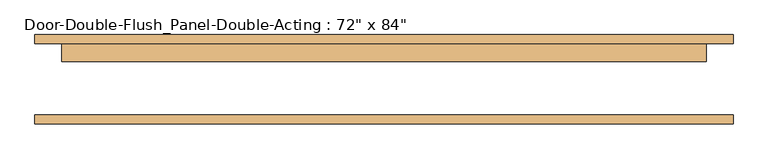
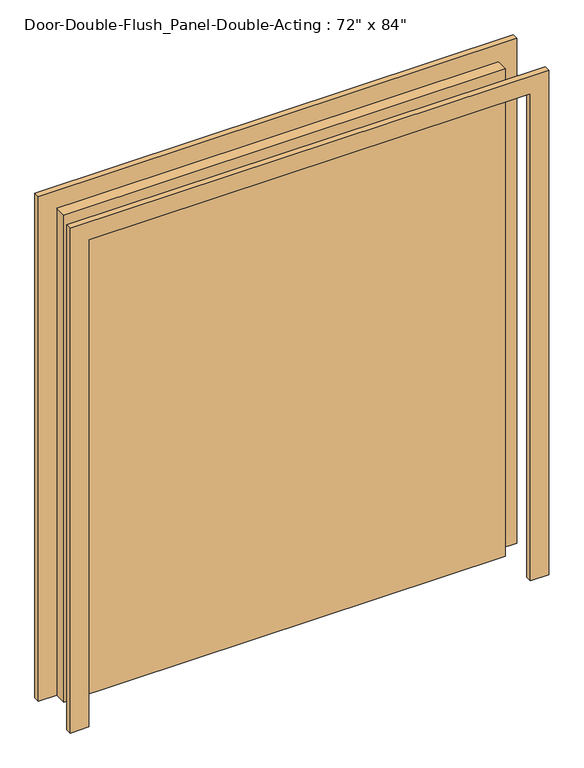
"""IFC4 building model written with IfcOpenShell, lengths in millimetres: door geometry."""

from ifc_helpers import new_model, si_unit, frame, origin, origin_with_axes, place, context, project, spatial, polyline, outline, extrude, source, transform, mapped, element, save


def door_4726f842(model_context):
    return source(origin(), model_context, "Body", "SweptSolid", [
        extrude(outline(polyline([(2209.8, -990.6), (0.0, -990.6), (0.0, -914.4), (2133.6, -914.4), (2133.6, 914.4), (0.0, 914.4), (0.0, 990.6), (2209.8, 990.6), (2209.8, -990.6)])), frame((0.0, 101.6, 0.0), z_axis=(0.0, 1.0, 0.0), x_axis=(0.0, 0.0, 1.0)), (0.0, 0.0, 1.0), 25.4),
        extrude(outline(polyline([(2133.6, -914.4), (2133.6, 914.4), (0.0, 914.4), (0.0, 990.6), (2209.8, 990.6), (2209.8, -990.6), (0.0, -990.6), (0.0, -914.4), (2133.6, -914.4)])), frame((0.0, -127.0, 0.0), z_axis=(0.0, 1.0, 0.0), x_axis=(0.0, 0.0, 1.0)), (0.0, 0.0, 1.0), 25.4),
        extrude(outline(polyline([(-914.4, 101.6), (914.4, 101.6), (914.4, 50.8), (-914.4, 50.8), (-914.4, 101.6)])), origin_with_axes(), (0.0, 0.0, 1.0), 2133.6),
    ])


if __name__ == "__main__":
    model = new_model("IFC4")
    model_context = context("Model", 3, world=origin())
    ifc_project = project(units=[si_unit("LENGTHUNIT", "METRE", prefix="MILLI")], contexts=[model_context])
    site = spatial("IfcSite", under=ifc_project)
    building = spatial("IfcBuilding", under=site)
    placement = place(None, origin())
    door_shape = door_4726f842(model_context)
    element("IfcDoor", 1, ObjectType="Door-Double-Flush_Panel-Double-Acting : 72\" x 84\"", at=placement, inside=building, context=model_context, shape_type="MappedRepresentation", body=[
        mapped(door_shape, transform((0.0, 0.0, 0.0), x_axis=(1.0, 0.0, 0.0), y_axis=(0.0, 1.0, 0.0), z_axis=(0.0, 0.0, 1.0))),
    ])
    save(model, "model.ifc")

# Revit data of these elements
# Type "Door-Double-Flush_Panel-Double-Acting : 72\" x 84\""
#   Type Mark = "10"
#   Construction Type Id = "DOOR"
#   Assembly Code = "C1020"
#   Analytic Construction = "Wooden"
#   W = 3' - 0"
#   Thickness = 0' - 2"
#   Thermal Resistance (R) = 0.455703 (m²·K)/W
#   Swing Angle [instance default] = 90.00°
#   Heat Transfer Coefficient (U) = 2.19465 W/(m²·K)
#   Height = 7' - 0"
#   Trim Projection Ext. = 0' - 1"
#   Trim Projection Int. = 0' - 1"
#   Trim Width Ext. = 0' - 3"
#   Trim Width Int. = 0' - 3"
#   Width = 6' - 0"
#   Panel Material = Wood - Birch - Solid Stained Light Low Gloss
#   Trim Material = Paint - Sienna
#   Visual Light Transmittance = 0
#   Solar Heat Gain Coefficient = 0
#   Function = (empty or 0)
#   Wall Closure = (empty or 0)
# Element 1 (IfcDoor, "Door-Double-Flush_Panel-Double-Acting : 72\" x 84\"")
#   Materials on its faces: "Paint - Sienna", "Wood - Birch - Solid Stained Light Low Gloss"
# Materials
#   "Wood - Birch - Solid Stained Light Low Gloss": class "Wood", colour RGB 210 159 95, transparency 0, Cost = 0
#   "Paint - Sienna": colour RGB 118 70 51, transparency 0, Cost = 0
